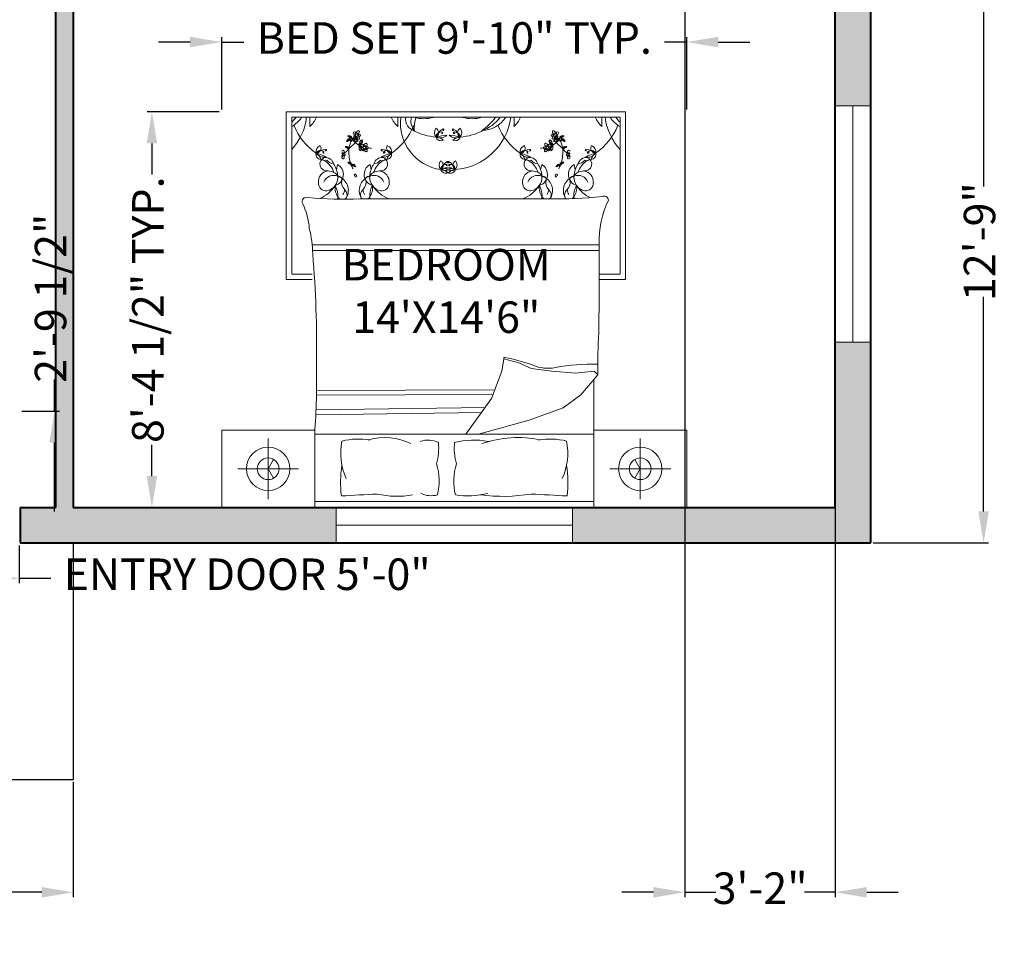
# Model space of a CAD drawing. Units: inches. Extents: x 2138 to 3265, y 2149 to 3392.
# Tile 2 of 13: x 2375 to 2625, y 2149 to 2382. Entities that reach past the tile are written whole.
import ezdxf

# ---------------------------------------------------------------- set-up
doc = ezdxf.new("R2010")
doc.units = ezdxf.units.IN
for name, color, linetype, lineweight in [('A-ANNO-DIMS', 2, 'Continuous', 18), ('A-AREA-IDEN', 7, 'Continuous', 18), ('A-FLOR', 7, 'Continuous', 25), ('A-FURN', 8, 'Continuous', 18), ('A-GLAZ', 150, 'Continuous', 18), ('A-WALL', 7, 'Continuous', 40), ('A-WALL-PATT', 142, 'Continuous', 13)]:
    doc.layers.add(name, color=color, linetype=linetype, lineweight=lineweight)
doc.styles.get("Standard").update_dxf_attribs({"font": 'arial.ttf'})
doc.dimstyles.new('ISO-25', dxfattribs={"dimtxt": 8, "dimasz": 8, "dimexe": 1.25, "dimexo": 0.625, "dimtad": 0, "dimdec": 1, "dimlunit": 4, "dimtxsty": 'Standard', "dimcen": 2.5, "dimadec": 0, "dimazin": 0, "dimtfac": 1, "dimtdec": 1, "dimtmove": 0, "dimatfit": 3, "dimfxl": 1, "dimarcsym": 0})

# ---------------------------------------------------------------- blocks, each defined once
blk = doc.blocks.new('bed')
for p, q in [((2648.79, 2367.17), (2766.9, 2367.17)), ((2672.41, 2367.17), (2672.41, 2334.75)), ((2743.28, 2365.66), (2672.41, 2365.66)), ((2660.6, 2349.61), (2660.6, 2365.05)), ((2755.09, 2349.61), (2755.09, 2365.05)), ((2668.32, 2357.33), (2652.88, 2357.33)), ((2747.37, 2357.33), (2762.8, 2357.33)), ((2672.41, 2348.51), (2743.28, 2348.51)), ((2688.82, 2345), (2701.7, 2348.51)), ((2704.86, 2348.51), (2698.39, 2339.5)), ((2680.2, 2341.89), (2688.82, 2345)), ((2742.96, 2343.6), (2700.91, 2343.01)), ((2675.66, 2338.54), (2680.2, 2341.89)), ((2742.91, 2342.39), (2700.03, 2341.78)), ((2671.35, 2333.52), (2675.66, 2338.54)), ((2698.39, 2339.5), (2695.75, 2332.57)), ((2742.85, 2338.67), (2698, 2338.49)), ((2742.86, 2337.46), (2697.54, 2337.27)), ((2672.31, 2332.57), (2671.35, 2333.52)), ((2677.09, 2333.04), (2672.31, 2332.57)), ((2683.08, 2332.57), (2677.09, 2333.04)), ((2688.34, 2331.85), (2683.08, 2332.57)), ((2691.45, 2330.41), (2688.34, 2331.85)), ((2695.28, 2329.46), (2691.45, 2330.41)), ((2695.75, 2332.57), (2695.28, 2329.46)), ((2664.38, 2309.27), (2671.06, 2309.27)), ((2664.38, 2266.73), (2664.38, 2309.27)), ((2671.06, 2307.91), (2665.75, 2307.91)), ((2665.75, 2307.91), (2665.75, 2268.1)), ((2749.12, 2307.91), (2743.91, 2307.91)), ((2743.94, 2309.27), (2750.49, 2309.27)), ((2749.12, 2268.1), (2749.12, 2307.91)), ((2750.49, 2309.27), (2750.49, 2266.73)), ((2743.81, 2301.91), (2671.05, 2301.91)), ((2743.93, 2300.44), (2671.05, 2300.44)), ((2731.82, 2288.83), (2683.87, 2288.83)), ((2677.39, 2280.07), (2677.12, 2281.41)), ((2685.64, 2280.07), (2685.9, 2281.41)), ((2729.22, 2280.07), (2728.96, 2281.41)), ((2737.48, 2280.07), (2737.74, 2281.41)), ((2665.75, 2268.1), (2749.12, 2268.1)), ((2750.49, 2266.73), (2664.38, 2266.73))]:
    blk.add_line(p, q)
for points in [[(2672.41, 2347.49), (2648.79, 2347.49), (2648.79, 2367.17)], [(2743.28, 2367.17), (2743.28, 2347.49), (2766.9, 2347.49), (2766.9, 2367.17)], [(2660.6, 2357.33), (2661.98, 2359.72)], [(2755.09, 2357.33), (2753.71, 2359.72)], [(2660.6, 2357.33), (2661.98, 2354.94)], [(2755.09, 2357.33), (2753.71, 2354.94)]]:
    blk.add_lwpolyline(points)
for points in [[(2679.19, 2364.23, 0.074897), (2679.34, 2356.51, -0.472817)], [(2707.29, 2356.08, 0.14099), (2707.53, 2363.95, 0.235245)], [(2712.33, 2356.08, -0.14099), (2712.1, 2363.95, -0.235245)], [(2736.49, 2364.23, -0.074897), (2736.35, 2356.51, 0.472817)], [(2671.11, 2322.71, 0.001242), (2671.05, 2300.3, -0.127202), (2668.68, 2289.13)], [(2743.78, 2302.84, 0.056112), (2744.64, 2296.34, 0.095341), (2746.3, 2290.08)]]:
    blk.add_lwpolyline(points, format="xyb")
for centre, radius in [((2660.6, 2357.33), 5.51), ((2755.09, 2357.33), 5.51), ((2660.6, 2357.33), 2.76), ((2755.09, 2357.33), 2.76), ((2684.21, 2275.79), 0.301), ((2730.65, 2275.79), 0.301), ((2682.24, 2272.62), 0.301), ((2732.62, 2272.62), 0.301)]:
    blk.add_circle(centre, radius)
for centre, radius, start, end in [((2744.3, 3488.25), 1125.9, 266.68521, 267.14978), ((2695.38, 2321.49), 42.84, 82.2196, 99.497), ((2704.43, 2343.14), 21.05, 81.5249, 103.96), ((2713.72, 2358.34), 5.84, 63.3437, 106.1026), ((2722.48, 2343.56), 20.76, 76.3427, 101.1841), ((2671.39, 3488.25), 1125.9, 272.85022, 273.31479), ((2694.24, 2353.42), 15.22, 155.1316, 191.7583), ((2721.45, 2353.42), 15.22, 348.2417, 24.8684), ((2693.37, 2352.14), 14.47, 354.0129, 15.8293), ((2726.26, 2352.14), 14.47, 164.1707, 185.9871), ((2683.41, 2365.61), 15.83, 255.1039, 281.0369), ((2691.74, 2376.86), 27.45, 258.0397, 289.2615), ((2702.85, 2370.87), 20.83, 259.8617, 283.6238), ((2714.51, 2356.3), 6.26, 245.0183, 288.5407), ((2725.45, 2364.44), 15.03, 243.8761, 286.1746), ((2732.28, 2365.61), 15.83, 258.9631, 284.8961), ((2955.01, 2334.07), 212.22, 176.1, 180.9282), ((2563.06, 2330.59), 108.33, 355.8294, 1.553), ((2673.37, 2375.35), 44.58, 267.4519, 281.3392), ((2684.03, 2322.21), 9.61, 66.2616, 101.3392), ((2703.48, 2374.09), 45.8, 250.1194, 259.3383), ((3019.62, 2326.36), 276.84, 179.1145, 184.8735), ((2695.01, 2329.36), 0.285, 268.8623, 19.7536), ((2669.77, 2289.2), 1.09, 183.98, 297.3412), ((2682.46, 2165.89), 122.95, 89.3433, 95.6887), ((2669.31, 2280.52), 8.94, 33.6671, 63.2997), ((2681.29, 2285.83), 4.56, 145.785, 184.7304), ((2672.59, 2287.96), 4.89, 328.8218, 9.1554), ((2678.65, 2287.53), 1.42, 120.0293, 142.325), ((2676.38, 2286.69), 3.76, 289.2822, 29.1751), ((2675.81, 2286.01), 3.4, 7.436, 29.9149), ((2678.05, 2287.81), 1.77, 311.5653, 23.8354), ((2678.65, 2287.53), 1.42, 44.4517, 63.558), ((2686.65, 2286.69), 3.76, 150.8249, 250.7178), ((2684.98, 2287.81), 1.77, 156.1646, 228.4347), ((2684.38, 2287.53), 1.42, 113.229, 135.5483), ((2687.22, 2286.01), 3.4, 150.0851, 172.564), ((2684.38, 2287.53), 1.42, 37.675, 66.7144), ((2681.74, 2285.83), 4.56, 355.2696, 34.215), ((2690.44, 2287.96), 4.89, 169.7133, 211.1782), ((2693.72, 2280.52), 8.94, 111.4941, 146.3329), ((2721.15, 2280.52), 8.94, 33.6671, 68.5059), ((2733.13, 2285.83), 4.56, 145.785, 184.7304), ((2724.42, 2287.96), 4.89, 328.8218, 10.2867), ((2730.49, 2287.53), 1.42, 113.2856, 142.325), ((2728.21, 2286.69), 3.76, 289.2822, 29.1751), ((2727.65, 2286.01), 3.4, 7.436, 29.9149), ((2730.49, 2287.53), 1.42, 44.4517, 66.7144), ((2729.88, 2287.81), 1.77, 311.5653, 23.8354), ((2735.44, 2173.96), 114.93, 85.2402, 91.8035), ((2738.49, 2286.69), 3.76, 150.8249, 250.7178), ((2736.82, 2287.81), 1.77, 156.1646, 228.4347), ((2736.22, 2287.53), 1.42, 106.6343, 135.5483), ((2739.05, 2286.01), 3.4, 150.0851, 172.564), ((2736.22, 2287.53), 1.42, 37.675, 72.5814), ((2733.57, 2285.83), 4.56, 355.2696, 34.215), ((2742.28, 2287.96), 4.89, 169.249, 211.1782), ((2745.56, 2280.52), 8.94, 113.6453, 146.3329), ((2745.4, 2289.48), 1.08, 246.5219, 33.8264), ((2674.52, 2284.81), 1.99, 84.4856, 181.0538), ((2673.9, 2283.33), 3.55, 355.2933, 76.921), ((2675.92, 2282.62), 2.94, 299.9085, 73.1337), ((2680.83, 2284.67), 2.42, 131.5653, 195.1471), ((2682.2, 2284.67), 2.42, 344.8529, 48.4347), ((2687.1, 2282.62), 2.94, 106.8663, 240.0915), ((2689.12, 2283.33), 3.55, 103.079, 184.7067), ((2688.51, 2284.81), 1.99, 358.9462, 95.5144), ((2726.35, 2284.81), 1.99, 84.4856, 181.0538), ((2725.74, 2283.33), 3.55, 355.2933, 76.921), ((2727.76, 2282.62), 2.94, 299.9085, 73.1337), ((2732.66, 2284.67), 2.42, 131.5653, 195.1471), ((2734.04, 2284.67), 2.42, 344.8529, 48.4347), ((2738.94, 2282.62), 2.94, 106.8663, 240.0915), ((2740.96, 2283.33), 3.55, 103.079, 184.7067), ((2740.35, 2284.81), 1.99, 358.9462, 95.5144), ((2675.33, 2284.52), 2.82, 174.9449, 262.8857), ((2676.44, 2285.59), 2.74, 201.5819, 291.4221), ((2674.84, 2285.15), 3.43, 272.3591, 324.0401), ((2671.12, 2283.43), 6.34, 326.2883, 356.5076), ((2681.29, 2285.83), 4.56, 212.7011, 216.3445), ((2677.78, 2283.85), 0.733, 257.3041, 15.1471), ((2681.85, 2282.74), 0.228, 102.7051, 280.4384), ((2681.83, 2282.88), 0.37, 280.4384, 100.4136), ((2685.25, 2283.85), 0.733, 164.8529, 282.6959), ((2681.74, 2285.83), 4.56, 323.6555, 327.2989), ((2688.18, 2285.15), 3.43, 215.9599, 267.6409), ((2686.58, 2285.59), 2.74, 248.5779, 338.4181), ((2691.91, 2283.43), 6.34, 183.4924, 213.7117), ((2687.69, 2284.52), 2.82, 277.1143, 5.0551), ((2727.17, 2284.52), 2.82, 174.9449, 262.8857), ((2728.28, 2285.59), 2.74, 201.5819, 291.4221), ((2726.68, 2285.15), 3.43, 272.3591, 324.0401), ((2722.96, 2283.43), 6.34, 326.2883, 356.5076), ((2733.13, 2285.83), 4.56, 212.7011, 216.3445), ((2729.62, 2283.85), 0.733, 257.3041, 15.1471), ((2733.04, 2282.88), 0.37, 79.5864, 259.5616), ((2733.01, 2282.74), 0.228, 259.5616, 77.2949), ((2737.08, 2283.85), 0.733, 164.8529, 282.6959), ((2733.57, 2285.83), 4.56, 323.6555, 327.2989), ((2740.02, 2285.15), 3.43, 215.9599, 267.6409), ((2738.42, 2285.59), 2.74, 248.5779, 338.4181), ((2743.75, 2283.43), 6.34, 183.4924, 213.7117), ((2739.53, 2284.52), 2.82, 277.1143, 5.0551), ((2674.68, 2279.97), 1.77, 80.264, 250.8688), ((2671.17, 2283.88), 5.58, 301.2614, 341.7045), ((2690.04, 2276.79), 9.78, 153.0032, 159.8941), ((2681.22, 2280.14), 0.241, 84.3784, 186.0543), ((2681, 2281.1), 0.99, 269.1859, 301.164), ((2681.29, 2280.59), 0.567, 237.5332, 323.4768), ((2680.74, 2282.21), 1.9, 285.5129, 293.6099), ((2681.98, 2280.07), 0.62, 87.3579, 140.4944), ((2680.54, 2281.85), 1.87, 301.164, 321.5612), ((2679.02, 2282.18), 3.33, 324.6898, 333.4936), ((2691.86, 2283.88), 5.58, 198.2955, 238.7386), ((2688.34, 2279.97), 1.77, 289.1312, 99.736), ((2708.76, 2266.02), 15.42, 94.4623, 172.255), ((2708.83, 2280.25), 1.71, 137.7873, 219.1145), ((2706.89, 2280.3), 1.29, 298.5391, 58.3627), ((2708.79, 2281.04), 1.28, 63.0274, 163.8037), ((2707.5, 2284.03), 2.63, 271.4585, 315.3727), ((2708.57, 2279.17), 2.44, 45.5411, 114.3101), ((2710.79, 2291.69), 10.79, 252.593, 267.2582), ((2708.82, 2281.35), 1.26, 177.7585, 283.852), ((2711.25, 2282.66), 3.9, 198.9159, 238.011), ((2710.23, 2279.17), 2.44, 65.6899, 134.4589), ((2708.01, 2291.69), 10.79, 272.7418, 287.407), ((2709.09, 2280.28), 0.167, 283.852, 219.9245), ((2710.01, 2281.04), 1.28, 16.1963, 116.9726), ((2711.31, 2284.03), 2.63, 224.6273, 268.5415), ((2709.7, 2280.35), 0.101, 320.1909, 256.0209), ((2707.55, 2282.66), 3.9, 301.989, 341.0841), ((2709.98, 2281.35), 1.26, 256.148, 2.2415), ((2711.91, 2280.3), 1.29, 121.6373, 241.4609), ((2709.97, 2280.25), 1.71, 320.8855, 42.2127), ((2709.54, 2269.58), 11.94, 352.8636, 81.8197), ((2726.52, 2279.97), 1.77, 80.264, 250.8688), ((2723.01, 2283.88), 5.58, 301.2614, 341.7045), ((2734.32, 2281.85), 1.87, 218.4388, 238.836), ((2732.89, 2280.07), 0.62, 39.5056, 92.6421), ((2735.84, 2282.18), 3.33, 206.5064, 215.3102), ((2733.58, 2280.59), 0.567, 216.5232, 302.4668), ((2733.87, 2281.1), 0.99, 238.836, 270.8141), ((2734.13, 2282.21), 1.9, 246.3901, 254.4871), ((2724.82, 2276.79), 9.78, 20.1059, 26.9968), ((2733.64, 2280.14), 0.241, 353.9457, 95.6216), ((2743.69, 2283.88), 5.58, 198.2955, 238.7386), ((2740.18, 2279.97), 1.77, 289.1312, 99.736), ((2673.18, 2277.52), 1.28, 92.9516, 193.728), ((2670.57, 2279.47), 2.63, 301.3827, 345.2969), ((2673.92, 2275.8), 2.44, 75.4653, 144.2343), ((2669.6, 2287.75), 10.79, 282.5173, 297.1824), ((2674.32, 2278.05), 1.09, 63.9755, 143.2681), ((2674.26, 2280.51), 2.21, 265.969, 344.3045), ((2676.64, 2277.57), 2.36, 96.1662, 141.5825), ((2678.79, 2278.04), 0.502, 101.5637, 142.6358), ((2678.38, 2277.58), 0.301, 273.2768, 86.7232), ((2678.73, 2277.86), 0.287, 91.1081, 181.8675), ((2679.03, 2277.29), 0.622, 80.3487, 133.6538), ((2678.39, 2278.44), 0.723, 288.7263, 352.5032), ((2678.88, 2278.4), 0.232, 345.2356, 144.9248), ((2679.1, 2277.64), 0.259, 317.6792, 80.3487), ((2680.55, 2279.22), 0.62, 101.3256, 154.4621), ((2679.66, 2281.32), 1.87, 280.2588, 300.656), ((2680.09, 2282.82), 3.33, 268.3264, 277.1302), ((2690.04, 2276.79), 9.78, 163.5842, 183.8277), ((2679.25, 2281.32), 1.9, 308.2101, 316.3071), ((2680.42, 2280.07), 0.567, 278.3432, 4.2869), ((2680.1, 2280.57), 0.99, 300.656, 332.6341), ((2680.85, 2279.92), 0.241, 55.7657, 157.4417), ((2686.38, 2277.57), 2.36, 38.4175, 83.8338), ((2688.77, 2280.51), 2.21, 195.6955, 274.031), ((2688.71, 2278.05), 1.09, 36.7319, 116.0245), ((2689.11, 2275.8), 2.44, 35.7657, 104.5347), ((2693.42, 2287.75), 10.79, 242.8176, 257.4827), ((2689.84, 2277.52), 1.28, 346.272, 87.0484), ((2692.46, 2279.47), 2.63, 194.7031, 238.6173), ((2709.29, 2279.51), 0.192, 238.011, 71.5592), ((2709.32, 2279.61), 0.093, 71.5592, 188.0167), ((2709.51, 2279.51), 0.192, 108.4408, 301.989), ((2709.48, 2279.61), 0.093, 351.9833, 108.4408), ((2725.02, 2277.52), 1.28, 92.9516, 193.728), ((2722.41, 2279.47), 2.63, 301.3827, 345.2969), ((2725.76, 2275.8), 2.44, 75.4653, 144.2343), ((2721.44, 2287.75), 10.79, 282.5173, 297.1824), ((2726.16, 2278.05), 1.09, 63.9755, 143.2681), ((2726.1, 2280.51), 2.21, 265.969, 344.3045), ((2728.48, 2277.57), 2.36, 96.1662, 141.5825), ((2734.02, 2279.92), 0.241, 22.5583, 124.2343), ((2734.45, 2280.07), 0.567, 175.7131, 261.6568), ((2734.76, 2280.57), 0.99, 207.3659, 239.344), ((2724.82, 2276.79), 9.78, 356.1723, 16.4158), ((2735.61, 2281.32), 1.9, 223.6929, 231.7899), ((2735.21, 2281.32), 1.87, 239.344, 259.7412), ((2734.78, 2282.82), 3.33, 262.8698, 271.6736), ((2734.32, 2279.22), 0.62, 25.5379, 78.6744), ((2735.77, 2277.64), 0.259, 99.6513, 222.3208), ((2735.83, 2277.29), 0.622, 46.3462, 99.6513), ((2735.98, 2278.4), 0.232, 35.0752, 194.7644), ((2736.47, 2278.44), 0.723, 187.4968, 251.2737), ((2736.13, 2277.86), 0.287, 358.1325, 88.8919), ((2736.07, 2278.04), 0.502, 37.3642, 78.4363), ((2736.49, 2277.58), 0.301, 93.2768, 266.7232), ((2740.6, 2280.51), 2.21, 195.6955, 274.031), ((2738.22, 2277.57), 2.36, 38.4175, 83.8338), ((2740.54, 2278.05), 1.09, 36.7319, 116.0245), ((2740.94, 2275.8), 2.44, 35.7657, 104.5347), ((2745.26, 2287.75), 10.79, 242.8176, 257.4827), ((2744.29, 2279.47), 2.63, 194.7031, 238.6173), ((2741.68, 2277.52), 1.28, 346.272, 87.0484), ((2654.26, 2266.02), 15.42, 7.745, 41.8856), ((2680.65, 2264.49), 15.42, 124.3865, 158.5908), ((2673.61, 2276.86), 1.71, 167.7115, 249.0387), ((2671.9, 2275.93), 1.29, 328.4633, 88.2869), ((2674.51, 2280.16), 3.9, 228.8402, 267.9352), ((2673.06, 2277.81), 1.26, 207.6827, 313.7762), ((2673.82, 2277.02), 0.167, 313.7762, 249.7183), ((2674.35, 2276.55), 0.093, 101.4834, 217.9409), ((2674.37, 2276.45), 0.192, 267.9352, 101.4834), ((2678.79, 2277.02), 0.497, 217.7621, 259.0403), ((2679.32, 2277.68), 0.913, 203.4276, 227.6104), ((2678.92, 2277.8), 0.492, 229.7889, 317.6792), ((2678.37, 2276.76), 0.699, 355.053, 68.3618), ((2678.92, 2276.64), 0.985, 83.0852, 105.7171), ((2678.83, 2276.72), 0.231, 232.4737, 355.053), ((2672.1, 2268.47), 11.21, 43.1541, 52.0459), ((2679.84, 2275.25), 0.62, 101.3256, 154.4621), ((2678.95, 2277.35), 1.87, 280.2588, 300.656), ((2679.38, 2278.84), 3.33, 268.3264, 277.1302), ((2678.55, 2277.34), 1.9, 308.2101, 316.3071), ((2679.71, 2276.1), 0.567, 278.3432, 4.2869), ((2679.4, 2276.6), 0.99, 300.656, 332.6341), ((2680.14, 2275.94), 0.241, 55.7657, 157.4417), ((2685.17, 2276.55), 4.9, 184.756, 209.2041), ((2692.23, 2286.99), 16.14, 222.2412, 232.1744), ((2681.91, 2276.24), 1.37, 304.5369, 16.3699), ((2682.64, 2275.93), 0.833, 272.8499, 356.1226), ((2682.05, 2275.61), 0.807, 321.7607, 7.9252), ((2683.81, 2275.85), 0.97, 127.3105, 187.9252), ((2682.48, 2275.96), 0.996, 355.0106, 41.658), ((2683.58, 2275.23), 0.298, 148.0499, 225.6268), ((2685.67, 2270.03), 5.88, 113.0501, 113.8477), ((2684.13, 2274.88), 0.948, 104.7558, 148.0499), ((2683.6, 2275.56), 0.594, 247.4086, 351.4386), ((2683.88, 2276.21), 0.41, 126.1046, 271.4281), ((2683.83, 2276.32), 0.295, 353.7526, 131.7054), ((2683.76, 2275.54), 0.199, 262.906, 7.132), ((2683.55, 2275.97), 0.414, 0.0645, 61.1507), ((2683.65, 2276.32), 0.473, 311.8413, 355.7877), ((2684.63, 2276.26), 0.502, 101.5637, 176.365), ((2684.62, 2275.23), 0.497, 151.2196, 259.0403), ((2684.56, 2276.08), 0.287, 91.1081, 181.8675), ((2685.16, 2275.9), 0.913, 203.4276, 227.6104), ((2684.87, 2275.5), 0.622, 80.3487, 133.6538), ((2684.75, 2276.01), 0.492, 229.7889, 317.6792), ((2684.22, 2276.65), 0.723, 288.7263, 352.5032), ((2684.2, 2274.97), 0.699, 355.053, 68.3618), ((2684.75, 2274.85), 0.985, 83.0852, 105.7171), ((2684.72, 2276.61), 0.232, 345.2356, 144.9248), ((2684.93, 2275.86), 0.259, 317.6792, 80.3487), ((2685.67, 2270.03), 5.88, 87.1071, 94.7585), ((2688.65, 2276.45), 0.192, 78.5166, 272.0648), ((2688.52, 2280.16), 3.9, 272.0648, 311.1598), ((2688.67, 2276.55), 0.093, 322.0591, 78.5166), ((2689.97, 2277.81), 1.26, 226.2238, 332.3173), ((2689.23, 2277.08), 0.101, 290.2667, 226.2271), ((2691.12, 2275.93), 1.29, 91.7131, 211.5367), ((2689.41, 2276.86), 1.71, 290.9613, 12.2885), ((2682.38, 2264.49), 15.42, 21.4092, 55.6135), ((2732.49, 2264.49), 15.42, 124.3865, 158.5908), ((2725.45, 2276.86), 1.71, 167.7115, 249.0387), ((2724.9, 2277.81), 1.26, 207.6827, 313.7762), ((2726.35, 2280.16), 3.9, 228.8402, 267.9352), ((2723.74, 2275.93), 1.29, 328.4633, 88.2869), ((2725.65, 2277.02), 0.167, 313.7762, 249.7183), ((2726.19, 2276.55), 0.093, 101.4834, 217.9409), ((2726.21, 2276.45), 0.192, 267.9352, 101.4834), ((2729.19, 2270.03), 5.88, 85.2415, 92.8929), ((2729.94, 2275.86), 0.259, 99.6513, 222.3208), ((2730.11, 2276.01), 0.492, 222.3208, 310.2111), ((2730, 2275.5), 0.622, 46.3462, 99.6513), ((2730.15, 2276.61), 0.232, 35.0752, 194.7644), ((2730.64, 2276.65), 0.723, 187.4968, 251.2737), ((2730.66, 2274.97), 0.699, 111.6382, 184.947), ((2730.12, 2274.85), 0.985, 74.2829, 96.9148), ((2730.3, 2276.08), 0.287, 358.1325, 88.8919), ((2729.71, 2275.9), 0.913, 312.3896, 336.5724), ((2730.24, 2276.26), 0.502, 3.635, 78.4363), ((2730.24, 2275.23), 0.497, 280.9597, 28.7804), ((2731.27, 2275.56), 0.594, 188.5614, 292.5914), ((2731.03, 2276.32), 0.295, 48.2946, 186.2474), ((2731.21, 2276.32), 0.473, 184.2123, 228.1587), ((2731.31, 2275.97), 0.414, 118.8493, 179.9355), ((2731.1, 2275.54), 0.199, 172.868, 277.094), ((2730.99, 2276.21), 0.41, 268.5719, 53.8954), ((2730.73, 2274.88), 0.948, 31.9501, 75.2442), ((2732.39, 2275.96), 0.996, 138.342, 184.9894), ((2732.22, 2275.93), 0.833, 183.8774, 267.1501), ((2731.29, 2275.23), 0.298, 314.3732, 31.9501), ((2729.19, 2270.03), 5.88, 66.1523, 66.9499), ((2732.96, 2276.24), 1.37, 163.6301, 235.4631), ((2731.05, 2275.85), 0.97, 352.0748, 52.6895), ((2732.81, 2275.61), 0.807, 172.0748, 218.2393), ((2722.64, 2286.99), 16.14, 307.8256, 317.7588), ((2729.7, 2276.55), 4.9, 330.7959, 355.244), ((2735.15, 2276.1), 0.567, 175.7131, 261.6568), ((2742.77, 2268.47), 11.21, 127.9541, 136.8459), ((2734.72, 2275.94), 0.241, 22.5583, 124.2343), ((2735.46, 2276.6), 0.99, 207.3659, 239.344), ((2736.32, 2277.34), 1.9, 223.6929, 231.7899), ((2735.91, 2277.35), 1.87, 239.344, 259.7412), ((2735.48, 2278.84), 3.33, 262.8698, 271.6736), ((2735.02, 2275.25), 0.62, 25.5379, 78.6744), ((2735.94, 2277.8), 0.492, 222.3208, 310.2111), ((2736.5, 2276.76), 0.699, 111.6382, 184.947), ((2736.03, 2276.72), 0.231, 184.947, 307.5263), ((2735.95, 2276.64), 0.985, 74.2829, 96.9148), ((2735.54, 2277.68), 0.913, 312.3896, 336.5724), ((2736.08, 2277.02), 0.497, 280.9597, 322.2379), ((2740.49, 2276.45), 0.192, 78.5166, 272.0648), ((2740.36, 2280.16), 3.9, 272.0648, 311.1598), ((2740.51, 2276.55), 0.093, 322.0591, 78.5166), ((2741.81, 2277.81), 1.26, 226.2238, 332.3173), ((2741.07, 2277.08), 0.101, 290.2667, 226.2271), ((2742.96, 2275.93), 1.29, 91.7131, 211.5367), ((2741.25, 2276.86), 1.71, 290.9613, 12.2885), ((2734.21, 2264.49), 15.42, 21.4092, 55.6135), ((2760.6, 2266.02), 15.42, 138.1144, 172.255), ((2680.05, 2274.16), 0.336, 146.8636, 236.9021), ((2684.79, 2281.56), 8.79, 235.1882, 238.8844), ((2680.63, 2274.64), 0.909, 199.4799, 267.6828), ((2680.53, 2274.3), 0.783, 212.8155, 277.3992), ((2680.07, 2273.78), 0.909, 266.9701, 338.2913), ((2675.28, 2280.27), 8.79, 302.6784, 306.3746), ((2680.3, 2273.06), 0.336, 214.3538, 304.3923), ((2680.43, 2274.33), 0.348, 238.8844, 314.2646), ((2680.35, 2273.55), 0.783, 280.3057, 17.1958), ((2680.29, 2273.47), 0.348, 306.3746, 21.7548), ((2680.85, 2273.7), 0.262, 19.3605, 201.7548), ((2680.85, 2273.89), 0.262, 311.8703, 134.2646), ((2685.79, 2271.5), 5.24, 153.7819, 158.2913), ((2681.62, 2275.08), 1.37, 247.2305, 319.0635), ((2681.16, 2274.62), 0.807, 264.4544, 310.6188), ((2685.17, 2276.55), 4.9, 214.0033, 222.4917), ((2681.75, 2274.3), 0.833, 218.3208, 298.8162), ((2685.67, 2270.03), 5.88, 120.544, 139.818), ((2681.91, 2273.04), 0.41, 126.1046, 271.4281), ((2681.86, 2273.15), 0.295, 353.7526, 131.7054), ((2682.32, 2273.27), 0.97, 70.0041, 130.6188), ((2681.59, 2272.8), 0.414, 0.0645, 61.1507), ((2681.69, 2273.15), 0.473, 311.8413, 355.7877), ((2681.69, 2274.45), 0.996, 297.7043, 344.3516), ((2682.66, 2273.09), 0.502, 101.5637, 176.365), ((2682.59, 2272.91), 0.287, 91.1081, 181.8675), ((2682.9, 2272.33), 0.622, 80.3487, 133.6538), ((2682.26, 2273.48), 0.723, 288.7263, 352.5032), ((2682.75, 2273.44), 0.232, 345.2356, 144.9248), ((2682.22, 2274.45), 0.807, 8.7227, 54.8872), ((2682.26, 2273.8), 1.37, 0.278, 72.111), ((2682.88, 2274.31), 0.833, 20.5253, 88.5375), ((2682.96, 2272.68), 0.259, 317.6792, 80.3487), ((2683.98, 2274.72), 0.97, 188.7227, 249.3375), ((2682.73, 2274.23), 0.996, 334.9899, 21.6373), ((2684.67, 2274.93), 0.231, 232.4737, 355.053), ((2707.58, 2257.76), 15.42, 94.4623, 117.4146), ((2707.65, 2271.98), 1.71, 137.7873, 219.1145), ((2705.71, 2272.04), 1.29, 298.5391, 58.3627), ((2707.61, 2272.78), 1.28, 63.0274, 163.8037), ((2706.31, 2275.77), 2.63, 271.4585, 315.3727), ((2707.39, 2270.91), 2.44, 45.5411, 114.3101), ((2710.07, 2274.4), 3.9, 198.9159, 238.011), ((2709.61, 2283.43), 10.79, 252.593, 267.2582), ((2707.64, 2273.08), 1.26, 177.7585, 283.852), ((2711.42, 2270.91), 2.44, 65.6899, 134.4589), ((2709.19, 2283.43), 10.79, 272.7418, 287.407), ((2711.19, 2272.78), 1.28, 16.1963, 116.9726), ((2712.49, 2275.77), 2.63, 224.6273, 268.5415), ((2708.73, 2274.4), 3.9, 301.989, 341.0841), ((2711.16, 2273.08), 1.26, 256.148, 2.2415), ((2713.1, 2272.04), 1.29, 121.6373, 241.4609), ((2711.15, 2271.98), 1.71, 320.8855, 42.2127), ((2711.22, 2257.76), 15.42, 62.5854, 85.5377), ((2730.2, 2274.93), 0.231, 184.947, 307.5263), ((2732.13, 2274.23), 0.996, 158.3627, 205.0101), ((2731.99, 2274.31), 0.833, 91.4625, 159.4747), ((2732.6, 2273.8), 1.37, 107.889, 179.722), ((2730.89, 2274.72), 0.97, 290.6625, 351.2773), ((2731.91, 2272.68), 0.259, 99.6513, 222.3208), ((2732.64, 2274.45), 0.807, 125.1128, 171.2773), ((2731.97, 2272.33), 0.622, 46.3462, 99.6513), ((2732.12, 2273.44), 0.232, 35.0752, 194.7644), ((2732.61, 2273.48), 0.723, 187.4968, 251.2737), ((2729.19, 2270.03), 5.88, 40.182, 59.456), ((2732.54, 2273.27), 0.97, 49.3812, 109.9959), ((2733.25, 2275.08), 1.37, 220.9365, 292.7695), ((2733.17, 2274.45), 0.996, 195.6484, 242.2957), ((2732.27, 2272.91), 0.287, 358.1325, 88.8919), ((2732.21, 2273.09), 0.502, 3.635, 78.4363), ((2733, 2273.15), 0.295, 48.2946, 186.2474), ((2733.11, 2274.3), 0.833, 241.1838, 321.6792), ((2733.18, 2273.15), 0.473, 184.2123, 228.1587), ((2733.28, 2272.8), 0.414, 118.8493, 179.9355), ((2732.95, 2273.04), 0.41, 268.5719, 53.8954), ((2733.7, 2274.62), 0.807, 229.3812, 275.5456), ((2729.7, 2276.55), 4.9, 317.5083, 325.9967), ((2734.51, 2273.55), 0.783, 162.8042, 259.6943), ((2734.01, 2273.89), 0.262, 45.7354, 228.1297), ((2734.01, 2273.7), 0.262, 338.2452, 160.6395), ((2729.08, 2271.5), 5.24, 21.7087, 26.2181), ((2734.79, 2273.78), 0.909, 201.7087, 273.0299), ((2734.44, 2274.33), 0.348, 225.7354, 301.1156), ((2734.34, 2274.3), 0.783, 262.6008, 327.1845), ((2734.58, 2273.47), 0.348, 158.2452, 233.6254), ((2734.23, 2274.64), 0.909, 272.3172, 340.5201), ((2739.58, 2280.27), 8.79, 233.6254, 237.3216), ((2734.56, 2273.06), 0.336, 235.6077, 325.6462), ((2730.07, 2281.56), 8.79, 301.1156, 304.8118), ((2734.81, 2274.16), 0.336, 303.0979, 33.1364), ((2662, 2263.95), 7.52, 33.4617, 60.1116), ((2666.21, 2265.69), 6.27, 22.5547, 48.9546), ((2649.03, 2269.06), 21.34, 357.4081, 3.6519), ((2681.61, 2272.06), 0.298, 148.0499, 225.6268), ((2682.16, 2271.71), 0.948, 104.7558, 148.0499), ((2681.63, 2272.39), 0.594, 247.4086, 351.4386), ((2681.8, 2272.37), 0.199, 262.906, 7.132), ((2682.65, 2272.06), 0.497, 151.2196, 259.0403), ((2683.19, 2272.72), 0.913, 203.4276, 227.6104), ((2682.79, 2272.84), 0.492, 229.7889, 317.6792), ((2682.23, 2271.8), 0.699, 355.053, 68.3618), ((2682.78, 2271.68), 0.985, 83.0852, 105.7171), ((2682.7, 2271.76), 0.231, 232.4737, 355.053), ((2696.82, 2265.69), 6.27, 131.0454, 157.4453), ((2713.99, 2269.06), 21.34, 176.3481, 182.5919), ((2701.02, 2263.95), 7.52, 91.272, 146.5383), ((2703.73, 2262.55), 9.37, 107.8504, 143.6964), ((2708.65, 2259.92), 13.93, 124.0123, 144.053), ((2707.9, 2272.02), 0.167, 283.852, 219.9245), ((2708.11, 2271.25), 0.192, 238.011, 71.5592), ((2708.14, 2271.35), 0.093, 71.5592, 188.0167), ((2710.69, 2271.25), 0.192, 108.4408, 301.989), ((2710.66, 2271.35), 0.093, 351.9833, 108.4408), ((2710.88, 2272.09), 0.101, 320.1909, 256.0209), ((2711.08, 2270.67), 6.91, 338.117, 6.6195), ((2717.42, 2268.75), 2.77, 346.3898, 79.0739), ((2715.34, 2269.13), 3.5, 342.8609, 41.9049), ((2700.87, 2269.06), 21.34, 357.4081, 3.6519), ((2718.05, 2265.69), 6.27, 22.5547, 48.9546), ((2732.08, 2272.84), 0.492, 222.3208, 310.2111), ((2732.63, 2271.8), 0.699, 111.6382, 184.947), ((2732.17, 2271.76), 0.231, 184.947, 307.5263), ((2732.08, 2271.68), 0.985, 74.2829, 96.9148), ((2731.68, 2272.72), 0.913, 312.3896, 336.5724), ((2732.21, 2272.06), 0.497, 280.9597, 28.7804), ((2733.23, 2272.39), 0.594, 188.5614, 292.5914), ((2733.07, 2272.37), 0.199, 172.868, 277.094), ((2732.7, 2271.71), 0.948, 31.9501, 75.2442), ((2733.25, 2272.06), 0.298, 314.3732, 31.9501), ((2748.65, 2265.69), 6.27, 131.0454, 157.4453), ((2765.83, 2269.06), 21.34, 176.3481, 182.5919), ((2752.86, 2263.95), 7.52, 119.8884, 146.5383), ((2659.3, 2262.55), 9.37, 36.3036, 46.4814), ((2703.27, 2259.99), 8.48, 73.5431, 107.0202), ((2706.63, 2255.62), 12.54, 94.3787, 95.6357), ((2713.23, 2247.02), 22.41, 109.7217, 109.9028), ((2715.53, 2259.99), 8.48, 72.9798, 106.4569), ((2712.17, 2255.62), 12.54, 84.3643, 85.6213), ((2705.57, 2247.02), 22.41, 70.0972, 70.2783), ((2755.57, 2262.55), 9.37, 133.5186, 143.6964)]:
    blk.add_arc(centre, radius, start, end)
blk = doc.blocks.new('GLAZ-SASH-60IN')
for p, q in [((0, 9), (0, 0)), ((60, 9), (60, 0)), ((0, 4.5), (60, 4.5))]:
    blk.add_line(p, q)
blk = doc.blocks.new('*D31')
at = {"layer": 'A-ANNO-DIMS', "color": 0, "lineweight": -2, "transparency": 16777216}
for p, q in [((2315.53, 2249.04), (2315.53, 2239.44)), ((2375.34, 2249.04), (2375.34, 2239.44)), ((2323.53, 2240.69), (2367.34, 2240.69)), ((2375.34, 2240.69), (2383.34, 2240.69))]:
    blk.add_line(p, q, dxfattribs=at)
at = {"layer": 'A-ANNO-DIMS', "color": 0, "transparency": 16777216}
for points in [[(2323.53, 2242.02), (2323.53, 2239.36), (2315.53, 2240.69)], [(2367.34, 2242.02), (2367.34, 2239.36), (2375.34, 2240.69)]]:
    blk.add_solid(points, dxfattribs=at)
at = {"layer": 'Defpoints', "color": 0, "transparency": 16777216}
for p in [(2315.53, 2249.66), (2375.34, 2249.66), (2375.34, 2240.69)]:
    blk.add_point(p, dxfattribs=at)
at = {"layer": 'A-ANNO-DIMS', "color": 0, "transparency": 16777216, "insert": (2433.19, 2240.69), "char_height": 8, "attachment_point": 5}
blk.add_mtext('ENTRY DOOR 5\'-0"', dxfattribs=at)
blk = doc.blocks.new('*D32')
at = {"layer": 'A-ANNO-DIMS', "color": 0, "lineweight": -2, "transparency": 16777216}
for p, q in [((2384.31, 2283.14), (2384.31, 2291.14)), ((2375.96, 2283.14), (2385.56, 2283.14)), ((2384.31, 2257.66), (2384.31, 2275.14)), ((2375.96, 2249.66), (2385.56, 2249.66))]:
    blk.add_line(p, q, dxfattribs=at)
at = {"layer": 'A-ANNO-DIMS', "color": 0, "transparency": 16777216}
for points in [[(2382.97, 2275.14), (2385.64, 2275.14), (2384.31, 2283.14)], [(2382.97, 2257.66), (2385.64, 2257.66), (2384.31, 2249.66)]]:
    blk.add_solid(points, dxfattribs=at)
at = {"layer": 'Defpoints', "color": 0, "transparency": 16777216}
for p in [(2375.34, 2283.14), (2384.31, 2283.14), (2375.34, 2249.66)]:
    blk.add_point(p, dxfattribs=at)
at = {"layer": 'A-ANNO-DIMS', "color": 0, "transparency": 16777216, "insert": (2384.31, 2311.79), "char_height": 8, "attachment_point": 5, "rotation": 90}
blk.add_mtext('2\'-9 1/2"', dxfattribs=at)
blk = doc.blocks.new('*D35')
at = {"layer": 'A-ANNO-DIMS', "color": 0, "lineweight": -2, "transparency": 16777216}
for p, q in [((2426.72, 2359.73), (2426.72, 2378.07)), ((2544.83, 2359.73), (2544.83, 2378.07)), ((2418.72, 2376.82), (2410.72, 2376.82)), ((2426.72, 2376.82), (2432.38, 2376.82)), ((2544.83, 2376.82), (2539.18, 2376.82)), ((2552.83, 2376.82), (2560.83, 2376.82))]:
    blk.add_line(p, q, dxfattribs=at)
at = {"layer": 'A-ANNO-DIMS', "color": 0, "transparency": 16777216}
for points in [[(2418.72, 2378.16), (2418.72, 2375.49), (2426.72, 2376.82)], [(2552.83, 2378.16), (2552.83, 2375.49), (2544.83, 2376.82)]]:
    blk.add_solid(points, dxfattribs=at)
at = {"layer": 'Defpoints', "color": 0, "transparency": 16777216}
for p in [(2426.72, 2376.82), (2426.72, 2359.11), (2544.83, 2359.11)]:
    blk.add_point(p, dxfattribs=at)
at = {"layer": 'A-ANNO-DIMS', "color": 0, "transparency": 16777216, "insert": (2485.78, 2376.82), "char_height": 8, "attachment_point": 5}
blk.add_mtext('BED SET 9\'-10" TYP.', dxfattribs=at)
blk = doc.blocks.new('*D36')
at = {"layer": 'A-ANNO-DIMS', "color": 0, "lineweight": -2, "transparency": 16777216}
for p, q in [((2426.1, 2359.11), (2407.76, 2359.11)), ((2409.01, 2351.11), (2409.01, 2343.22)), ((2409.01, 2266.66), (2409.01, 2274.55)), ((2426.1, 2258.66), (2407.76, 2258.66))]:
    blk.add_line(p, q, dxfattribs=at)
at = {"layer": 'A-ANNO-DIMS', "color": 0, "transparency": 16777216}
for points in [[(2407.67, 2351.11), (2410.34, 2351.11), (2409.01, 2359.11)], [(2407.67, 2266.66), (2410.34, 2266.66), (2409.01, 2258.66)]]:
    blk.add_solid(points, dxfattribs=at)
at = {"layer": 'Defpoints', "color": 0, "transparency": 16777216}
for p in [(2426.72, 2359.11), (2409.01, 2258.66), (2426.72, 2258.66)]:
    blk.add_point(p, dxfattribs=at)
at = {"layer": 'A-ANNO-DIMS', "color": 0, "transparency": 16777216, "insert": (2409.01, 2308.88), "char_height": 8, "attachment_point": 5, "rotation": 90}
blk.add_mtext('8\'-4 1/2" TYP.', dxfattribs=at)
blk = doc.blocks.new('*D52')
at = {"layer": 'A-ANNO-DIMS', "color": 0, "lineweight": -2, "transparency": 16777216}
for p, q in [((2207.53, 2189.04), (2207.53, 2159.74)), ((2389.03, 2189.04), (2389.03, 2159.74)), ((2215.53, 2160.99), (2274.97, 2160.99)), ((2381.03, 2160.99), (2321.59, 2160.99))]:
    blk.add_line(p, q, dxfattribs=at)
at = {"layer": 'A-ANNO-DIMS', "color": 0, "transparency": 16777216}
for points in [[(2215.53, 2162.32), (2215.53, 2159.65), (2207.53, 2160.99)], [(2381.03, 2162.32), (2381.03, 2159.65), (2389.03, 2160.99)]]:
    blk.add_solid(points, dxfattribs=at)
at = {"layer": 'Defpoints', "color": 0, "transparency": 16777216}
for p in [(2207.53, 2189.66), (2389.03, 2189.66), (2389.03, 2160.99)]:
    blk.add_point(p, dxfattribs=at)
at = {"layer": 'A-ANNO-DIMS', "color": 0, "transparency": 16777216, "insert": (2298.28, 2160.99), "char_height": 8, "attachment_point": 5}
blk.add_mtext('15\'-1 1/2"', dxfattribs=at)
blk = doc.blocks.new('*D56')
at = {"layer": 'A-ANNO-DIMS', "color": 0, "lineweight": -2, "transparency": 16777216}
for p, q in [((2583.15, 2402.66), (2621.45, 2402.66)), ((2620.2, 2394.66), (2620.2, 2340.15)), ((2620.2, 2257.66), (2620.2, 2312.17)), ((2592.15, 2249.66), (2621.45, 2249.66))]:
    blk.add_line(p, q, dxfattribs=at)
at = {"layer": 'A-ANNO-DIMS', "color": 0, "transparency": 16777216}
for points in [[(2618.87, 2394.66), (2621.54, 2394.66), (2620.2, 2402.66)], [(2618.87, 2257.66), (2621.54, 2257.66), (2620.2, 2249.66)]]:
    blk.add_solid(points, dxfattribs=at)
at = {"layer": 'Defpoints', "color": 0, "transparency": 16777216}
for p in [(2582.53, 2402.66), (2620.2, 2402.66), (2591.53, 2249.66)]:
    blk.add_point(p, dxfattribs=at)
at = {"layer": 'A-ANNO-DIMS', "color": 0, "transparency": 16777216, "insert": (2620.2, 2326.16), "char_height": 8, "attachment_point": 5, "rotation": 90}
blk.add_mtext('12\'-9"', dxfattribs=at)
blk = doc.blocks.new('*D58')
at = {"layer": 'A-ANNO-DIMS', "color": 0, "lineweight": -2, "transparency": 16777216}
for p, q in [((2544.36, 2720.04), (2544.36, 2159.74)), ((2582.53, 2720.04), (2582.53, 2159.74)), ((2536.36, 2160.99), (2528.36, 2160.99)), ((2544.36, 2160.99), (2552.19, 2160.99)), ((2582.53, 2160.99), (2574.7, 2160.99)), ((2590.53, 2160.99), (2598.53, 2160.99))]:
    blk.add_line(p, q, dxfattribs=at)
at = {"layer": 'A-ANNO-DIMS', "color": 0, "transparency": 16777216}
for points in [[(2536.36, 2162.32), (2536.36, 2159.65), (2544.36, 2160.99)], [(2590.53, 2162.32), (2590.53, 2159.65), (2582.53, 2160.99)]]:
    blk.add_solid(points, dxfattribs=at)
at = {"layer": 'Defpoints', "color": 0, "transparency": 16777216}
for p in [(2544.36, 2720.66), (2582.53, 2720.66), (2544.36, 2160.99)]:
    blk.add_point(p, dxfattribs=at)
at = {"layer": 'A-ANNO-DIMS', "color": 0, "transparency": 16777216, "insert": (2563.45, 2160.99), "char_height": 8, "attachment_point": 5}
blk.add_mtext('3\'-2"', dxfattribs=at)
blk = doc.blocks.new('*D60')
at = {"layer": 'A-ANNO-DIMS', "color": 0, "lineweight": -2, "transparency": 16777216}
for p, q in [((2178.85, 2427.16), (2178.85, 2435.16)), ((2493.4, 2419.16), (2177.6, 2419.16)), ((2178.85, 2419.16), (2178.85, 2402.66)), ((2493.4, 2402.66), (2177.6, 2402.66)), ((2178.85, 2394.66), (2178.85, 2386.66))]:
    blk.add_line(p, q, dxfattribs=at)
at = {"layer": 'A-ANNO-DIMS', "color": 0, "transparency": 16777216}
for points in [[(2177.52, 2427.16), (2180.19, 2427.16), (2178.85, 2419.16)], [(2177.52, 2394.66), (2180.19, 2394.66), (2178.85, 2402.66)]]:
    blk.add_solid(points, dxfattribs=at)
at = {"layer": 'Defpoints', "color": 0, "transparency": 16777216}
for p in [(2494.03, 2419.16), (2178.85, 2402.66), (2494.03, 2402.66)]:
    blk.add_point(p, dxfattribs=at)
at = {"layer": 'A-ANNO-DIMS', "color": 0, "transparency": 16777216, "insert": (2178.85, 2366.46), "char_height": 8, "attachment_point": 5, "rotation": 90}
blk.add_mtext('1\'-4 1/2"', dxfattribs=at)

msp = doc.modelspace()

# ---------------------------------------------------------------- hatches: boundary and pattern name
at = {"layer": 'A-WALL-PATT'}
h = msp.add_hatch(color=256, dxfattribs=at)
h.dxf.hatch_style = 1
h.paths.add_polyline_path([(2270.53, 2729.66), (2207.53, 2729.66), (2207.53, 2663.66), (2216.53, 2663.66), (2216.53, 2720.66), (2270.53, 2720.66)])
h.paths.add_polyline_path([(2484.36, 2729.66), (2330.53, 2729.66), (2330.53, 2720.66), (2384.53, 2720.66), (2384.53, 2546.66), (2372.53, 2546.66), (2372.53, 2542.16), (2389.03, 2542.16), (2389.03, 2720.66), (2484.36, 2720.66)])
h.paths.add_polyline_path([(2591.53, 2729.66), (2544.36, 2729.66), (2544.36, 2720.66), (2582.53, 2720.66), (2582.53, 2684.66), (2591.53, 2684.66)])
h.paths.add_polyline_path([(2591.53, 2624.66), (2582.53, 2624.66), (2582.53, 2588.66), (2456.53, 2588.66), (2456.53, 2584.16), (2582.53, 2584.16), (2582.53, 2512.16), (2456.53, 2512.16), (2456.53, 2507.66), (2494.03, 2507.66), (2494.03, 2501.66), (2498.53, 2501.66), (2498.53, 2507.66), (2582.53, 2507.66), (2582.53, 2495.66), (2591.53, 2495.66)])
h.paths.add_polyline_path([(2591.53, 2471.66), (2582.53, 2471.66), (2582.53, 2459.66), (2498.53, 2459.66), (2498.53, 2471.66), (2497.72, 2471.66, -0.030629), (2494.03, 2471.44), (2494.03, 2459.66), (2431.08, 2459.66, -0.013128), (2431.03, 2457.77), (2431.03, 2455.16), (2494.03, 2455.16), (2494.03, 2449.16), (2498.53, 2449.16), (2498.53, 2455.16), (2582.53, 2455.16), (2582.53, 2443.16), (2591.53, 2443.16)])
h.paths.add_polyline_path([(2591.53, 2419.16), (2582.53, 2419.16), (2582.53, 2407.16), (2498.53, 2407.16), (2498.53, 2419.16), (2497.72, 2419.16, -0.030629), (2494.03, 2418.94), (2494.03, 2402.66), (2582.53, 2402.66), (2582.53, 2360.66), (2591.53, 2360.66)])
h.paths.add_polyline_path([(2591.53, 2300.66), (2582.53, 2300.66), (2582.53, 2258.66), (2515.78, 2258.66), (2515.78, 2249.66), (2591.53, 2249.66)])
h.paths.add_polyline_path([(2455.78, 2258.66), (2389.03, 2258.66), (2389.03, 2455.16), (2395.03, 2455.16), (2395.03, 2459.66), (2384.53, 2459.66), (2384.53, 2258.66), (2375.53, 2258.66), (2375.53, 2249.66), (2455.78, 2249.66)])
h.paths.add_polyline_path([(2315.53, 2253.24), (2315.53, 2258.66), (2296.03, 2258.66), (2296.03, 2249.66), (2315.53, 2249.66)])
h.paths.add_polyline_path([(2236.03, 2258.66), (2216.53, 2258.66), (2216.53, 2290.16), (2207.53, 2290.16), (2207.53, 2249.66), (2236.03, 2249.66)])
h.paths.add_polyline_path([(2216.53, 2396.66), (2207.53, 2396.66), (2207.53, 2350.16), (2216.53, 2350.16)])
h.paths.add_polyline_path([(2216.53, 2603.66), (2207.53, 2603.66), (2207.53, 2456.66), (2216.53, 2456.66), (2216.53, 2542.16), (2264.53, 2542.16), (2264.53, 2470.16), (2252.53, 2470.16), (2252.53, 2465.66), (2269.03, 2465.66), (2269.03, 2542.16), (2336.48, 2542.16, -0.013128), (2336.53, 2544.05), (2336.53, 2546.66), (2216.53, 2546.66)])

# ---------------------------------------------------------------- linework, layer by layer
at = {"layer": 'A-FLOR'}
for p in [(2389.03, 2249.66), (2207.53, 2189.66)]:
    msp.add_line(p, (2389.03, 2189.66), dxfattribs=at)
at = {"layer": 'A-GLAZ'}
for p, q in [((2455.78, 2258.66), (2455.78, 2249.66)), ((2515.78, 2258.66), (2515.78, 2249.66))]:
    msp.add_line(p, q, dxfattribs=at)
for points in [[(2582.53, 2360.66), (2591.53, 2360.66), (2591.53, 2300.66), (2582.53, 2300.66)], [(2455.78, 2258.66), (2515.78, 2258.66), (2515.78, 2249.66), (2455.78, 2249.66)], [(2515.78, 2254.16), (2455.78, 2254.16), (2455.78, 2254.16), (2515.78, 2254.16)]]:
    msp.add_lwpolyline(points, close=True, dxfattribs=at)
at = {"layer": 'A-WALL'}
for p, q in [((2591.53, 2249.66), (2591.53, 2729.66)), ((2384.53, 2459.66), (2384.53, 2258.66)), ((2389.03, 2455.16), (2389.03, 2258.66)), ((2582.53, 2258.66), (2582.53, 2402.66)), ((2375.53, 2258.66), (2375.53, 2249.66)), ((2375.53, 2258.66), (2384.53, 2258.66)), ((2389.03, 2258.66), (2582.53, 2258.66)), ((2375.53, 2249.66), (2591.53, 2249.66))]:
    msp.add_line(p, q, dxfattribs=at)

# ---------------------------------------------------------------- block references
at = {"layer": 'A-FURN', "rotation": 180}
msp.add_blockref('bed', (5193.62, 4625.83), dxfattribs=at)
at = {"layer": 'A-GLAZ', "rotation": 89.99999999999916}
msp.add_blockref('GLAZ-SASH-60IN', (2591.53, 2300.66), dxfattribs=at)

# ---------------------------------------------------------------- texts
at = {"layer": 'A-AREA-IDEN', "insert": (2445.23, 2324.31), "char_height": 8, "attachment_point": 1}
msp.add_mtext_dynamic_manual_height_columns('\\pxqc;BEDROOM\\P14\'X14\'6"', width=77.0226, gutter_width=12.5, heights=[0], dxfattribs=at)

# ---------------------------------------------------------------- dimensions: what is measured, and where the dimension line sits
at = {"layer": 'A-ANNO-DIMS'}
for base, p1, p2, picture, middle in [((2544.36, 2160.99), (2582.53, 2720.66), (2544.36, 2720.66), '*D58', (2563.45, 2160.99)), ((2389.03, 2160.99), (2207.53, 2189.66), (2389.03, 2189.66), '*D52', (2298.28, 2160.99))]:
    dim = msp.add_linear_dim(base=base, p1=p1, p2=p2, dimstyle='ISO-25', override={"dimdec": 1, "dimlfac": 1, "dimrnd": 0, "dimzin": 1, "dimdsep": 46, "dimlunit": 4, "dimfrac": 2}, dxfattribs=at)
    dim.commit()
    dim.dimension.update_dxf_attribs({"geometry": picture, "text_midpoint": middle})
for base, p1, p2, picture, middle in [((2178.85, 2402.66), (2494.03, 2419.16), (2494.03, 2402.66), '*D60', (2178.85, 2366.46)), ((2620.2, 2402.66), (2591.53, 2249.66), (2582.53, 2402.66), '*D56', (2620.2, 2326.16)), ((2384.31, 2283.14), (2375.34, 2249.66), (2375.34, 2283.14), '*D32', (2384.31, 2311.79))]:
    dim = msp.add_linear_dim(base=base, p1=p1, p2=p2, angle=90, dimstyle='ISO-25', override={"dimdec": 1, "dimlfac": 1, "dimrnd": 0, "dimzin": 1, "dimdsep": 46, "dimlunit": 4, "dimfrac": 2}, dxfattribs=at)
    dim.commit()
    dim.dimension.update_dxf_attribs({"geometry": picture, "text_midpoint": middle})
for base, p1, p2, angle, text, picture, middle in [((2426.72, 2376.82), (2544.83, 2359.11), (2426.72, 2359.11), 180, 'BED SET <> TYP.', '*D35', (2485.78, 2376.82)), ((2409.0079, 2258.6616), (2426.7244, 2359.1063), (2426.7244, 2258.6616), 270, '<> TYP.', '*D36', (2409.0079, 2308.8839))]:
    dim = msp.add_linear_dim(base=base, p1=p1, p2=p2, angle=angle, text=text, dimstyle='ISO-25', override={"dimdec": 1, "dimlfac": 1, "dimrnd": 0, "dimzin": 1, "dimdsep": 46, "dimlunit": 4, "dimfrac": 2}, dxfattribs=at)
    dim.commit()
    dim.dimension.update_dxf_attribs({"geometry": picture, "text_midpoint": middle})
dim = msp.add_linear_dim(base=(2375.34, 2240.69), p1=(2315.53, 2249.66), p2=(2375.34, 2249.66), text='ENTRY DOOR <>', dimstyle='ISO-25', override={"dimdec": 1, "dimlfac": 1, "dimrnd": 0, "dimzin": 1, "dimdsep": 46, "dimlunit": 4, "dimfrac": 2}, dxfattribs=at)
dim.commit()
dim.dimension.update_dxf_attribs({"geometry": '*D31', "text_midpoint": (2433.19, 2240.69)})

doc.saveas('drawing.dxf')
